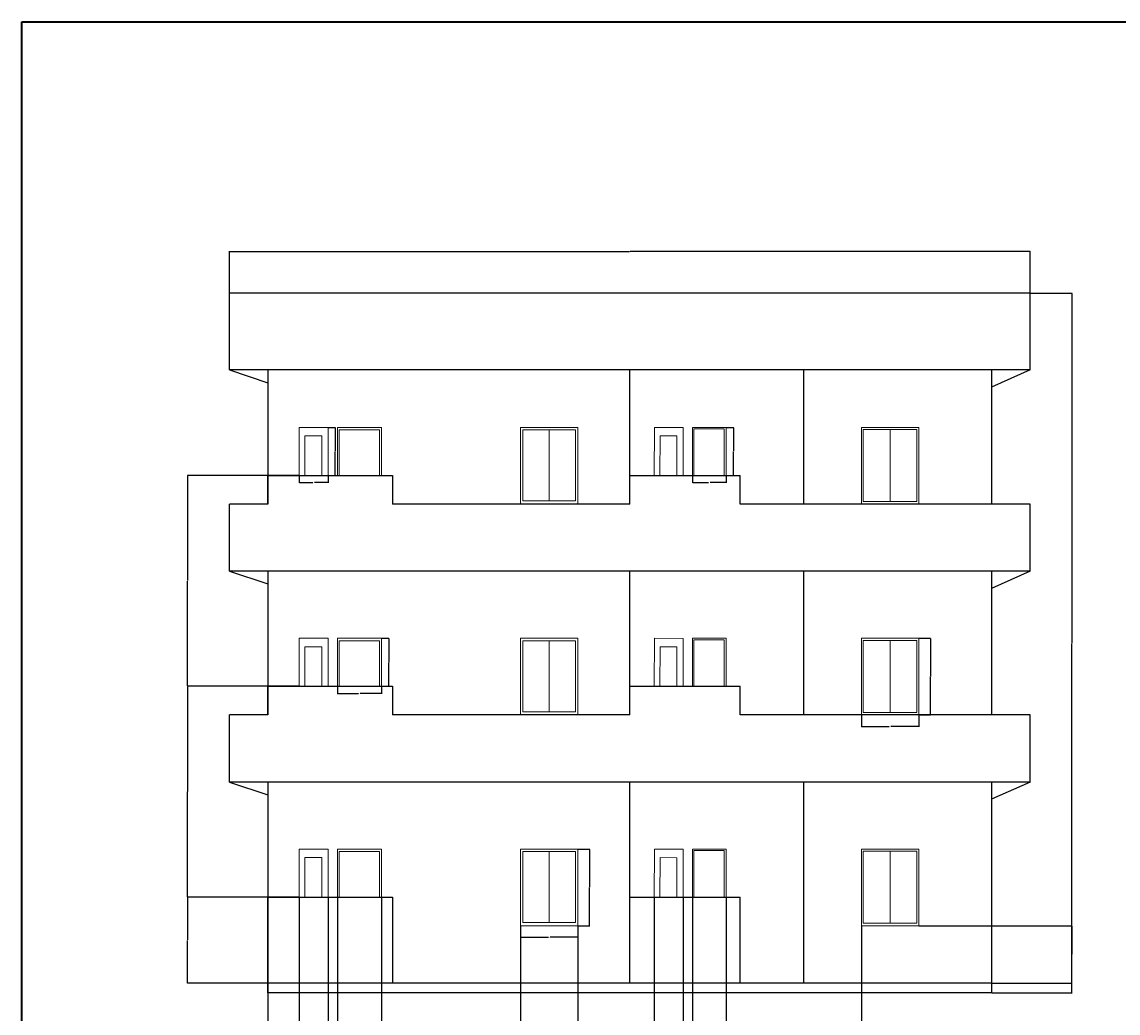
# Model space of a CAD drawing. Units: inches. Extents: x 2250 to 3629, y 982 to 2740.
# Tile 11 of 12: x 2250 to 2936, y 2119 to 2740. Entities that reach past the tile are written whole.
import ezdxf

# ---------------------------------------------------------------- set-up
doc = ezdxf.new("R2010")
doc.units = ezdxf.units.IN
for name, color, linetype, lineweight in [('A-ANNO-DIMS', 2, 'Continuous', 18), ('A-ANNO-TTLB', 7, 'Continuous', 35), ('A-ELEV', 7, 'Continuous', 25), ('A-ELEV-DOOR', 3, 'Continuous', 18), ('A-ELEV-GLAZ', 4, 'Continuous', 18)]:
    doc.layers.add(name, color=color, linetype=linetype, lineweight=lineweight)
doc.styles.get("Standard").update_dxf_attribs({"font": 'arial.ttf'})
doc.dimstyles.get("Standard").update_dxf_attribs({"dimtxt": 0.18, "dimasz": 0.18, "dimexe": 0.18, "dimexo": 0.0625, "dimgap": 0.09, "dimtad": 0, "dimtih": 1, "dimtoh": 1, "dimdec": 4, "dimzin": 0, "dimdsep": 46, "dimtxsty": 'Standard', "dimcen": 0.09, "dimadec": 0, "dimazin": 0, "dimtfac": 1, "dimtdec": 4, "dimtofl": 0, "dimtmove": 0, "dimatfit": 3, "dimfxl": 1, "dimtolj": 1, "dimtzin": 0, "dimarcsym": 0})

# ---------------------------------------------------------------- blocks, each defined once
blk = doc.blocks.new('EL-DOOR-18p04x30')
for p, q in [((0, 30), (0, 0)), ((18.04, 30), (0, 30)), ((18.04, 30), (18.04, 0))]:
    blk.add_line(p, q)
blk.add_lwpolyline([(3.53, 0), (3.53, 24.67), (14.13, 24.67), (14.13, 0)])
blk = doc.blocks.new('EL-WIN-27p64x30')
for p, q in [((0, 30), (0, 0)), ((27.64, 30), (0, 30)), ((27.64, 30), (27.64, 0))]:
    blk.add_line(p, q)
blk.add_lwpolyline([(1.16, 0), (1.16, 28.46), (26.36, 28.46), (26.36, 0)])
blk = doc.blocks.new('EL-WIN-36x48-A')
for p, q in [((0, 48), (0, 0)), ((36, 48), (0, 48)), ((17.95, 2), (17.95, 46.41)), ((36, 48), (36, 0)), ((36, 0), (0, 0))]:
    blk.add_line(p, q)
blk.add_lwpolyline([(1.44, 46.41), (34.46, 46.41), (34.46, 2), (1.44, 2)], close=True)
blk = doc.blocks.new('EL-WIN-21p24x30')
for p, q in [((0, 30), (0, 0)), ((21.23, 30), (0, 30)), ((0, 0), (0, 30)), ((21.23, 30), (21.23, 0)), ((21.23, 0), (21.23, 30))]:
    blk.add_line(p, q)
blk.add_lwpolyline([(0.82, 0), (0.82, 29.09), (19.98, 29.09), (19.98, 0)])
blk = doc.blocks.new('EL-WIN-36x48-B')
for p, q in [((0, 48), (0, 0)), ((36, 48), (0, 48)), ((17.97, 1.54), (17.97, 46.64)), ((36, 48), (36, 0)), ((36, 0), (0, 0))]:
    blk.add_line(p, q)
blk.add_lwpolyline([(1.24, 46.64), (34.71, 46.64), (34.71, 1.54), (1.24, 1.54)], close=True)
blk = doc.blocks.new('*D147')
at = {"layer": 'A-ANNO-DIMS', "color": 0, "lineweight": -2, "transparency": 16777216}
for p, q in [((2441.39, 2485.7), (2446.01, 2485.7)), ((2445.83, 2485.52), (2445.83, 2470.88)), ((2445.83, 2455.88), (2445.83, 2470.52)), ((2441.39, 2455.7), (2446.01, 2455.7))]:
    blk.add_line(p, q, dxfattribs=at)
at = {"layer": 'A-ANNO-DIMS', "color": 0, "transparency": 16777216}
for points in [[(2445.8, 2485.52), (2445.86, 2485.52), (2445.83, 2485.7)], [(2445.8, 2455.88), (2445.86, 2455.88), (2445.83, 2455.7)]]:
    blk.add_solid(points, dxfattribs=at)
at = {"layer": 'Defpoints', "color": 0, "transparency": 16777216}
for p in [(2441.33, 2485.7), (2445.83, 2485.7), (2441.33, 2455.7)]:
    blk.add_point(p, dxfattribs=at)
at = {"layer": 'A-ANNO-DIMS', "color": 0, "transparency": 16777216, "insert": (2445.83, 2470.7), "char_height": 0.18, "attachment_point": 5}
blk.add_mtext('\\A1;DOOR 30 TYP.', dxfattribs=at)
blk = doc.blocks.new('*D148')
at = {"layer": 'A-ANNO-DIMS', "color": 0, "lineweight": -2, "transparency": 16777216}
for p, q in [((2423.28, 2455.64), (2423.28, 2451.02)), ((2423.46, 2451.2), (2431.78, 2451.2)), ((2441.15, 2451.2), (2432.82, 2451.2)), ((2441.33, 2455.64), (2441.33, 2451.02))]:
    blk.add_line(p, q, dxfattribs=at)
at = {"layer": 'A-ANNO-DIMS', "color": 0, "transparency": 16777216}
for points in [[(2423.46, 2451.23), (2423.46, 2451.17), (2423.28, 2451.2)], [(2441.15, 2451.23), (2441.15, 2451.17), (2441.33, 2451.2)]]:
    blk.add_solid(points, dxfattribs=at)
at = {"layer": 'Defpoints', "color": 0, "transparency": 16777216}
for p in [(2423.28, 2455.7), (2441.33, 2455.7), (2441.33, 2451.2)]:
    blk.add_point(p, dxfattribs=at)
at = {"layer": 'A-ANNO-DIMS', "color": 0, "transparency": 16777216, "insert": (2432.3, 2451.2), "char_height": 0.18, "attachment_point": 5}
blk.add_mtext('\\A1;18 TYP.', dxfattribs=at)
blk = doc.blocks.new('*D149')
at = {"layer": 'A-ANNO-DIMS', "color": 0, "lineweight": -2, "transparency": 16777216}
for p, q in [((2474.81, 2353.7), (2479.42, 2353.7)), ((2479.24, 2353.52), (2479.24, 2338.88)), ((2479.24, 2323.88), (2479.24, 2338.52)), ((2474.81, 2323.7), (2479.42, 2323.7))]:
    blk.add_line(p, q, dxfattribs=at)
at = {"layer": 'A-ANNO-DIMS', "color": 0, "transparency": 16777216}
for points in [[(2479.21, 2353.52), (2479.27, 2353.52), (2479.24, 2353.7)], [(2479.21, 2323.88), (2479.27, 2323.88), (2479.24, 2323.7)]]:
    blk.add_solid(points, dxfattribs=at)
at = {"layer": 'Defpoints', "color": 0, "transparency": 16777216}
for p in [(2474.74, 2353.7), (2479.24, 2353.7), (2474.74, 2323.7)]:
    blk.add_point(p, dxfattribs=at)
at = {"layer": 'A-ANNO-DIMS', "color": 0, "transparency": 16777216, "insert": (2479.24, 2338.7), "char_height": 0.18, "attachment_point": 5}
blk.add_mtext('\\A1;WINDOW 30 TYP.', dxfattribs=at)
blk = doc.blocks.new('*D150')
at = {"layer": 'A-ANNO-DIMS', "color": 0, "lineweight": -2, "transparency": 16777216}
for p, q in [((2447.11, 2323.64), (2447.11, 2319.02)), ((2447.29, 2319.2), (2460.4, 2319.2)), ((2474.56, 2319.2), (2461.46, 2319.2)), ((2474.74, 2323.64), (2474.74, 2319.02))]:
    blk.add_line(p, q, dxfattribs=at)
at = {"layer": 'A-ANNO-DIMS', "color": 0, "transparency": 16777216}
for points in [[(2447.29, 2319.23), (2447.29, 2319.17), (2447.11, 2319.2)], [(2474.56, 2319.23), (2474.56, 2319.17), (2474.74, 2319.2)]]:
    blk.add_solid(points, dxfattribs=at)
at = {"layer": 'Defpoints', "color": 0, "transparency": 16777216}
for p in [(2447.11, 2323.7), (2474.74, 2323.7), (2474.74, 2319.2)]:
    blk.add_point(p, dxfattribs=at)
at = {"layer": 'A-ANNO-DIMS', "color": 0, "transparency": 16777216, "insert": (2460.93, 2319.2), "char_height": 0.18, "attachment_point": 5}
blk.add_mtext('\\A1;28 TYP.', dxfattribs=at)
blk = doc.blocks.new('*D151')
at = {"layer": 'A-ANNO-DIMS', "color": 0, "lineweight": -2, "transparency": 16777216}
for p, q in [((2597.75, 2221.7), (2605.07, 2221.7)), ((2604.89, 2221.52), (2604.89, 2197.88)), ((2604.89, 2173.88), (2604.89, 2197.52)), ((2597.75, 2173.7), (2605.07, 2173.7))]:
    blk.add_line(p, q, dxfattribs=at)
at = {"layer": 'A-ANNO-DIMS', "color": 0, "transparency": 16777216}
for points in [[(2604.86, 2221.52), (2604.92, 2221.52), (2604.89, 2221.7)], [(2604.86, 2173.88), (2604.92, 2173.88), (2604.89, 2173.7)]]:
    blk.add_solid(points, dxfattribs=at)
at = {"layer": 'Defpoints', "color": 0, "transparency": 16777216}
for p in [(2597.69, 2221.7), (2604.89, 2221.7), (2597.69, 2173.7)]:
    blk.add_point(p, dxfattribs=at)
at = {"layer": 'A-ANNO-DIMS', "color": 0, "transparency": 16777216, "insert": (2604.89, 2197.7), "char_height": 0.18, "attachment_point": 5}
blk.add_mtext('\\A1;WINDOW 48 TYP.', dxfattribs=at)
blk = doc.blocks.new('*D152')
at = {"layer": 'A-ANNO-DIMS', "color": 0, "lineweight": -2, "transparency": 16777216}
for p, q in [((2561.69, 2173.64), (2561.69, 2166.32)), ((2597.69, 2173.64), (2597.69, 2166.32)), ((2561.87, 2166.5), (2579.16, 2166.5)), ((2597.51, 2166.5), (2580.22, 2166.5))]:
    blk.add_line(p, q, dxfattribs=at)
at = {"layer": 'A-ANNO-DIMS', "color": 0, "transparency": 16777216}
for points in [[(2561.87, 2166.53), (2561.87, 2166.47), (2561.69, 2166.5)], [(2597.51, 2166.53), (2597.51, 2166.47), (2597.69, 2166.5)]]:
    blk.add_solid(points, dxfattribs=at)
at = {"layer": 'Defpoints', "color": 0, "transparency": 16777216}
for p in [(2561.69, 2173.7), (2597.69, 2173.7), (2597.69, 2166.5)]:
    blk.add_point(p, dxfattribs=at)
at = {"layer": 'A-ANNO-DIMS', "color": 0, "transparency": 16777216, "insert": (2579.69, 2166.5), "char_height": 0.18, "attachment_point": 5}
blk.add_mtext('\\A1;36 TYP.', dxfattribs=at)
blk = doc.blocks.new('*D153')
at = {"layer": 'A-ANNO-DIMS', "color": 0, "lineweight": -2, "transparency": 16777216}
for p, q in [((2690.61, 2485.7), (2695.22, 2485.7)), ((2695.04, 2485.52), (2695.04, 2470.88)), ((2695.04, 2455.88), (2695.04, 2470.52)), ((2690.61, 2455.7), (2695.22, 2455.7))]:
    blk.add_line(p, q, dxfattribs=at)
at = {"layer": 'A-ANNO-DIMS', "color": 0, "transparency": 16777216}
for points in [[(2695.01, 2485.52), (2695.07, 2485.52), (2695.04, 2485.7)], [(2695.01, 2455.88), (2695.07, 2455.88), (2695.04, 2455.7)]]:
    blk.add_solid(points, dxfattribs=at)
at = {"layer": 'Defpoints', "color": 0, "transparency": 16777216}
for p in [(2690.54, 2485.7), (2695.04, 2485.7), (2690.54, 2455.7)]:
    blk.add_point(p, dxfattribs=at)
at = {"layer": 'A-ANNO-DIMS', "color": 0, "transparency": 16777216, "insert": (2695.04, 2470.7), "char_height": 0.18, "attachment_point": 5}
blk.add_mtext('\\A1;WINDOW 30 TYP.', dxfattribs=at)
blk = doc.blocks.new('*D154')
at = {"layer": 'A-ANNO-DIMS', "color": 0, "lineweight": -2, "transparency": 16777216}
for p, q in [((2669.31, 2455.64), (2669.31, 2451.02)), ((2669.49, 2451.2), (2679.4, 2451.2)), ((2690.36, 2451.2), (2680.46, 2451.2)), ((2690.54, 2455.64), (2690.54, 2451.02))]:
    blk.add_line(p, q, dxfattribs=at)
at = {"layer": 'A-ANNO-DIMS', "color": 0, "transparency": 16777216}
for points in [[(2669.49, 2451.23), (2669.49, 2451.17), (2669.31, 2451.2)], [(2690.36, 2451.23), (2690.36, 2451.17), (2690.54, 2451.2)]]:
    blk.add_solid(points, dxfattribs=at)
at = {"layer": 'Defpoints', "color": 0, "transparency": 16777216}
for p in [(2669.31, 2455.7), (2690.54, 2455.7), (2690.54, 2451.2)]:
    blk.add_point(p, dxfattribs=at)
at = {"layer": 'A-ANNO-DIMS', "color": 0, "transparency": 16777216, "insert": (2679.93, 2451.2), "char_height": 0.18, "attachment_point": 5}
blk.add_mtext('\\A1;21 TYP.', dxfattribs=at)
blk = doc.blocks.new('*D155')
at = {"layer": 'A-ANNO-DIMS', "color": 0, "lineweight": -2, "transparency": 16777216}
for p, q in [((2811.11, 2353.7), (2818.43, 2353.7)), ((2818.25, 2353.52), (2818.25, 2329.88)), ((2818.25, 2305.88), (2818.25, 2329.52)), ((2811.11, 2305.7), (2818.43, 2305.7))]:
    blk.add_line(p, q, dxfattribs=at)
at = {"layer": 'A-ANNO-DIMS', "color": 0, "transparency": 16777216}
for points in [[(2818.22, 2353.52), (2818.28, 2353.52), (2818.25, 2353.7)], [(2818.22, 2305.88), (2818.28, 2305.88), (2818.25, 2305.7)]]:
    blk.add_solid(points, dxfattribs=at)
at = {"layer": 'Defpoints', "color": 0, "transparency": 16777216}
for p in [(2811.05, 2353.7), (2818.25, 2353.7), (2811.05, 2305.7)]:
    blk.add_point(p, dxfattribs=at)
at = {"layer": 'A-ANNO-DIMS', "color": 0, "transparency": 16777216, "insert": (2818.25, 2329.7), "char_height": 0.18, "attachment_point": 5}
blk.add_mtext('\\A1;WINDOW 48 TYP.', dxfattribs=at)
blk = doc.blocks.new('*D156')
at = {"layer": 'A-ANNO-DIMS', "color": 0, "lineweight": -2, "transparency": 16777216}
for p, q in [((2775.05, 2305.64), (2775.05, 2298.32)), ((2811.05, 2305.64), (2811.05, 2298.32)), ((2775.23, 2298.5), (2792.52, 2298.5)), ((2810.87, 2298.5), (2793.58, 2298.5))]:
    blk.add_line(p, q, dxfattribs=at)
at = {"layer": 'A-ANNO-DIMS', "color": 0, "transparency": 16777216}
for points in [[(2775.23, 2298.53), (2775.23, 2298.47), (2775.05, 2298.5)], [(2810.87, 2298.53), (2810.87, 2298.47), (2811.05, 2298.5)]]:
    blk.add_solid(points, dxfattribs=at)
at = {"layer": 'Defpoints', "color": 0, "transparency": 16777216}
for p in [(2775.05, 2305.7), (2811.05, 2305.7), (2811.05, 2298.5)]:
    blk.add_point(p, dxfattribs=at)
at = {"layer": 'A-ANNO-DIMS', "color": 0, "transparency": 16777216, "insert": (2793.05, 2298.5), "char_height": 0.18, "attachment_point": 5}
blk.add_mtext('\\A1;36 TYP.', dxfattribs=at)
blk = doc.blocks.new('*D176')
at = {"layer": 'A-ANNO-DIMS', "color": 0, "lineweight": -2, "transparency": 16777216}
for p, q in [((2379.61, 2569.76), (2379.61, 2596.08)), ((2379.79, 2595.9), (2629.84, 2595.9)), ((2880.43, 2595.9), (2630.38, 2595.9)), ((2880.61, 2569.76), (2880.61, 2596.08))]:
    blk.add_line(p, q, dxfattribs=at)
at = {"layer": 'A-ANNO-DIMS', "color": 0, "transparency": 16777216}
for points in [[(2379.79, 2595.93), (2379.79, 2595.87), (2379.61, 2595.9)], [(2880.43, 2595.93), (2880.43, 2595.87), (2880.61, 2595.9)]]:
    blk.add_solid(points, dxfattribs=at)
at = {"layer": 'Defpoints', "color": 0, "transparency": 16777216}
for p in [(2880.61, 2595.9), (2379.61, 2569.7), (2880.61, 2569.7)]:
    blk.add_point(p, dxfattribs=at)
at = {"layer": 'A-ANNO-DIMS', "color": 0, "transparency": 16777216, "insert": (2630.11, 2595.9), "char_height": 0.18, "attachment_point": 5}
blk.add_mtext('\\A1;501', dxfattribs=at)
blk = doc.blocks.new('*D177')
at = {"layer": 'A-ANNO-DIMS', "color": 0, "lineweight": -2, "transparency": 16777216}
for p, q in [((2880.67, 2569.7), (2906.99, 2569.7)), ((2906.81, 2569.52), (2906.81, 2350.88)), ((2906.81, 2131.88), (2906.81, 2350.52)), ((2856.67, 2131.7), (2906.99, 2131.7))]:
    blk.add_line(p, q, dxfattribs=at)
at = {"layer": 'A-ANNO-DIMS', "color": 0, "transparency": 16777216}
for points in [[(2906.78, 2569.52), (2906.84, 2569.52), (2906.81, 2569.7)], [(2906.78, 2131.88), (2906.84, 2131.88), (2906.81, 2131.7)]]:
    blk.add_solid(points, dxfattribs=at)
at = {"layer": 'Defpoints', "color": 0, "transparency": 16777216}
for p in [(2880.61, 2569.7), (2906.81, 2569.7), (2856.61, 2131.7)]:
    blk.add_point(p, dxfattribs=at)
at = {"layer": 'A-ANNO-DIMS', "color": 0, "transparency": 16777216, "insert": (2906.81, 2350.7), "char_height": 0.18, "attachment_point": 5}
blk.add_mtext('\\A1;438', dxfattribs=at)
blk = doc.blocks.new('*D178')
at = {"layer": 'A-ANNO-DIMS', "color": 0, "lineweight": -2, "transparency": 16777216}
for p, q in [((2423.22, 2191.7), (2353.23, 2191.7)), ((2353.41, 2191.52), (2353.41, 2164.88)), ((2353.41, 2137.88), (2353.41, 2164.52)), ((2403.54, 2137.7), (2353.23, 2137.7))]:
    blk.add_line(p, q, dxfattribs=at)
at = {"layer": 'A-ANNO-DIMS', "color": 0, "transparency": 16777216}
for points in [[(2353.38, 2191.52), (2353.44, 2191.52), (2353.41, 2191.7)], [(2353.38, 2137.88), (2353.44, 2137.88), (2353.41, 2137.7)]]:
    blk.add_solid(points, dxfattribs=at)
at = {"layer": 'Defpoints', "color": 0, "transparency": 16777216}
for p in [(2353.41, 2191.7), (2423.28, 2191.7), (2403.61, 2137.7)]:
    blk.add_point(p, dxfattribs=at)
at = {"layer": 'A-ANNO-DIMS', "color": 0, "transparency": 16777216, "insert": (2353.41, 2164.7), "char_height": 0.18, "attachment_point": 5}
blk.add_mtext('\\A1;54', dxfattribs=at)
blk = doc.blocks.new('*D179')
at = {"layer": 'A-ANNO-DIMS', "color": 0, "lineweight": -2, "transparency": 16777216}
for p, q in [((2423.22, 2323.7), (2353.23, 2323.7)), ((2353.41, 2323.52), (2353.41, 2257.88)), ((2353.41, 2191.88), (2353.41, 2257.52)), ((2423.22, 2191.7), (2353.23, 2191.7))]:
    blk.add_line(p, q, dxfattribs=at)
at = {"layer": 'A-ANNO-DIMS', "color": 0, "transparency": 16777216}
for points in [[(2353.38, 2323.52), (2353.44, 2323.52), (2353.41, 2323.7)], [(2353.38, 2191.88), (2353.44, 2191.88), (2353.41, 2191.7)]]:
    blk.add_solid(points, dxfattribs=at)
at = {"layer": 'Defpoints', "color": 0, "transparency": 16777216}
for p in [(2353.41, 2323.7), (2423.28, 2323.7), (2423.28, 2191.7)]:
    blk.add_point(p, dxfattribs=at)
at = {"layer": 'A-ANNO-DIMS', "color": 0, "transparency": 16777216, "insert": (2353.41, 2257.7), "char_height": 0.18, "attachment_point": 5}
blk.add_mtext('\\A1;132', dxfattribs=at)
blk = doc.blocks.new('*D180')
at = {"layer": 'A-ANNO-DIMS', "color": 0, "lineweight": -2, "transparency": 16777216}
for p, q in [((2423.22, 2455.7), (2353.23, 2455.7)), ((2353.41, 2455.52), (2353.41, 2389.88)), ((2353.41, 2323.88), (2353.41, 2389.52)), ((2423.22, 2323.7), (2353.23, 2323.7))]:
    blk.add_line(p, q, dxfattribs=at)
at = {"layer": 'A-ANNO-DIMS', "color": 0, "transparency": 16777216}
for points in [[(2353.38, 2455.52), (2353.44, 2455.52), (2353.41, 2455.7)], [(2353.38, 2323.88), (2353.44, 2323.88), (2353.41, 2323.7)]]:
    blk.add_solid(points, dxfattribs=at)
at = {"layer": 'Defpoints', "color": 0, "transparency": 16777216}
for p in [(2353.41, 2455.7), (2423.28, 2455.7), (2423.28, 2323.7)]:
    blk.add_point(p, dxfattribs=at)
at = {"layer": 'A-ANNO-DIMS', "color": 0, "transparency": 16777216, "insert": (2353.41, 2389.7), "char_height": 0.18, "attachment_point": 5}
blk.add_mtext('\\A1;132', dxfattribs=at)
blk = doc.blocks.new('*D181')
at = {"layer": 'A-ANNO-DIMS', "color": 0, "lineweight": -2, "transparency": 16777216}
for p, q in [((2423.28, 2191.64), (2423.28, 2061.34)), ((2403.61, 2131.64), (2403.61, 2061.34)), ((2403.79, 2061.52), (2412.99, 2061.52)), ((2423.1, 2061.52), (2413.9, 2061.52))]:
    blk.add_line(p, q, dxfattribs=at)
at = {"layer": 'A-ANNO-DIMS', "color": 0, "transparency": 16777216}
for points in [[(2403.79, 2061.55), (2403.79, 2061.49), (2403.61, 2061.52)], [(2423.1, 2061.55), (2423.1, 2061.49), (2423.28, 2061.52)]]:
    blk.add_solid(points, dxfattribs=at)
at = {"layer": 'Defpoints', "color": 0, "transparency": 16777216}
for p in [(2423.28, 2191.7), (2403.61, 2131.7), (2423.28, 2061.52)]:
    blk.add_point(p, dxfattribs=at)
at = {"layer": 'A-ANNO-DIMS', "color": 0, "transparency": 16777216, "insert": (2413.44, 2061.52), "char_height": 0.18, "attachment_point": 5}
blk.add_mtext('\\A1;19.674', dxfattribs=at)
blk = doc.blocks.new('*D182')
at = {"layer": 'A-ANNO-DIMS', "color": 0, "lineweight": -2, "transparency": 16777216}
for p, q in [((2441.33, 2191.64), (2441.33, 2061.34)), ((2447.11, 2191.64), (2447.11, 2061.34)), ((2441.51, 2061.52), (2443.84, 2061.52)), ((2446.93, 2061.52), (2444.59, 2061.52))]:
    blk.add_line(p, q, dxfattribs=at)
at = {"layer": 'A-ANNO-DIMS', "color": 0, "transparency": 16777216}
for points in [[(2441.51, 2061.55), (2441.51, 2061.49), (2441.33, 2061.52)], [(2446.93, 2061.55), (2446.93, 2061.49), (2447.11, 2061.52)]]:
    blk.add_solid(points, dxfattribs=at)
at = {"layer": 'Defpoints', "color": 0, "transparency": 16777216}
for p in [(2441.33, 2191.7), (2447.11, 2191.7), (2447.11, 2061.52)]:
    blk.add_point(p, dxfattribs=at)
at = {"layer": 'A-ANNO-DIMS', "color": 0, "transparency": 16777216, "insert": (2444.22, 2061.52), "char_height": 0.18, "attachment_point": 5}
blk.add_mtext('\\A1;5.781', dxfattribs=at)
blk = doc.blocks.new('*D183')
at = {"layer": 'A-ANNO-DIMS', "color": 0, "lineweight": -2, "transparency": 16777216}
for p, q in [((2474.74, 2191.64), (2474.74, 2061.34)), ((2561.69, 2173.64), (2561.69, 2061.34)), ((2474.92, 2061.52), (2517.82, 2061.52)), ((2561.51, 2061.52), (2518.61, 2061.52))]:
    blk.add_line(p, q, dxfattribs=at)
at = {"layer": 'A-ANNO-DIMS', "color": 0, "transparency": 16777216}
for points in [[(2474.92, 2061.55), (2474.92, 2061.49), (2474.74, 2061.52)], [(2561.51, 2061.55), (2561.51, 2061.49), (2561.69, 2061.52)]]:
    blk.add_solid(points, dxfattribs=at)
at = {"layer": 'Defpoints', "color": 0, "transparency": 16777216}
for p in [(2474.74, 2191.7), (2561.69, 2173.7), (2561.69, 2061.52)]:
    blk.add_point(p, dxfattribs=at)
at = {"layer": 'A-ANNO-DIMS', "color": 0, "transparency": 16777216, "insert": (2518.22, 2061.52), "char_height": 0.18, "attachment_point": 5}
blk.add_mtext('\\A1;86.94', dxfattribs=at)
blk = doc.blocks.new('*D184')
at = {"layer": 'A-ANNO-DIMS', "color": 0, "lineweight": -2, "transparency": 16777216}
for p, q in [((2645.41, 2191.68), (2645.41, 2061.34)), ((2597.69, 2173.64), (2597.69, 2061.34)), ((2597.87, 2061.52), (2621.08, 2061.52)), ((2645.23, 2061.52), (2622.02, 2061.52))]:
    blk.add_line(p, q, dxfattribs=at)
at = {"layer": 'A-ANNO-DIMS', "color": 0, "transparency": 16777216}
for points in [[(2597.87, 2061.55), (2597.87, 2061.49), (2597.69, 2061.52)], [(2645.23, 2061.55), (2645.23, 2061.49), (2645.41, 2061.52)]]:
    blk.add_solid(points, dxfattribs=at)
at = {"layer": 'Defpoints', "color": 0, "transparency": 16777216}
for p in [(2645.41, 2191.74), (2597.69, 2173.7), (2645.41, 2061.52)]:
    blk.add_point(p, dxfattribs=at)
at = {"layer": 'A-ANNO-DIMS', "color": 0, "transparency": 16777216, "insert": (2621.55, 2061.52), "char_height": 0.18, "attachment_point": 5}
blk.add_mtext('\\A1;47.725', dxfattribs=at)
blk = doc.blocks.new('*D185')
at = {"layer": 'A-ANNO-DIMS', "color": 0, "lineweight": -2, "transparency": 16777216}
for p, q in [((2663.46, 2191.6), (2663.46, 2061.34)), ((2669.31, 2191.64), (2669.31, 2061.34)), ((2663.64, 2061.52), (2666.06, 2061.52)), ((2669.13, 2061.52), (2666.71, 2061.52))]:
    blk.add_line(p, q, dxfattribs=at)
at = {"layer": 'A-ANNO-DIMS', "color": 0, "transparency": 16777216}
for points in [[(2663.64, 2061.55), (2663.64, 2061.49), (2663.46, 2061.52)], [(2669.13, 2061.55), (2669.13, 2061.49), (2669.31, 2061.52)]]:
    blk.add_solid(points, dxfattribs=at)
at = {"layer": 'Defpoints', "color": 0, "transparency": 16777216}
for p in [(2663.46, 2191.66), (2669.31, 2191.7), (2669.31, 2061.52)]:
    blk.add_point(p, dxfattribs=at)
at = {"layer": 'A-ANNO-DIMS', "color": 0, "transparency": 16777216, "insert": (2666.38, 2061.52), "char_height": 0.18, "attachment_point": 5}
blk.add_mtext('\\A1;5.85', dxfattribs=at)
blk = doc.blocks.new('*D186')
at = {"layer": 'A-ANNO-DIMS', "color": 0, "lineweight": -2, "transparency": 16777216}
for p, q in [((2690.54, 2191.64), (2690.54, 2061.34)), ((2775.05, 2173.64), (2775.05, 2061.34)), ((2690.72, 2061.52), (2732.47, 2061.52)), ((2774.87, 2061.52), (2733.12, 2061.52))]:
    blk.add_line(p, q, dxfattribs=at)
at = {"layer": 'A-ANNO-DIMS', "color": 0, "transparency": 16777216}
for points in [[(2690.72, 2061.55), (2690.72, 2061.49), (2690.54, 2061.52)], [(2774.87, 2061.55), (2774.87, 2061.49), (2775.05, 2061.52)]]:
    blk.add_solid(points, dxfattribs=at)
at = {"layer": 'Defpoints', "color": 0, "transparency": 16777216}
for p in [(2690.54, 2191.7), (2775.05, 2173.7), (2775.05, 2061.52)]:
    blk.add_point(p, dxfattribs=at)
at = {"layer": 'A-ANNO-DIMS', "color": 0, "transparency": 16777216, "insert": (2732.8, 2061.52), "char_height": 0.18, "attachment_point": 5}
blk.add_mtext('\\A1;84.5', dxfattribs=at)
blk = doc.blocks.new('*D187')
at = {"layer": 'A-ANNO-DIMS', "color": 0, "lineweight": -2, "transparency": 16777216}
for p, q in [((2811.11, 2173.7), (2906.99, 2173.7)), ((2906.81, 2173.52), (2906.81, 2155.88)), ((2906.81, 2137.88), (2906.81, 2155.52)), ((2856.67, 2137.7), (2906.99, 2137.7))]:
    blk.add_line(p, q, dxfattribs=at)
at = {"layer": 'A-ANNO-DIMS', "color": 0, "transparency": 16777216}
for points in [[(2906.78, 2173.52), (2906.84, 2173.52), (2906.81, 2173.7)], [(2906.78, 2137.88), (2906.84, 2137.88), (2906.81, 2137.7)]]:
    blk.add_solid(points, dxfattribs=at)
at = {"layer": 'Defpoints', "color": 0, "transparency": 16777216}
for p in [(2811.05, 2173.7), (2906.81, 2173.7), (2856.61, 2137.7)]:
    blk.add_point(p, dxfattribs=at)
at = {"layer": 'A-ANNO-DIMS', "color": 0, "transparency": 16777216, "insert": (2906.81, 2155.7), "char_height": 0.18, "attachment_point": 5}
blk.add_mtext('\\A1;36', dxfattribs=at)

msp = doc.modelspace()

# ---------------------------------------------------------------- linework, layer by layer
at = {"layer": 'A-ANNO-TTLB'}
msp.add_lwpolyline([(2249.6849, 2739.593), (3629.4532, 2739.593), (3629.4532, 982.3108), (2249.6849, 982.3108)], close=True, dxfattribs=at)
at = {"layer": 'A-ELEV'}
for p, q in [((2880.6072, 2569.6999), (2379.6072, 2569.6999)), ((2379.6072, 2521.6999), (2379.6072, 2569.6999)), ((2880.6072, 2521.6999), (2880.6072, 2569.6999)), ((2880.6072, 2521.6999), (2379.6072, 2521.6999)), ((2379.6072, 2521.6999), (2403.6072, 2513.7231)), ((2403.6072, 2521.6999), (2403.6072, 2437.6999)), ((2630.1072, 2437.6999), (2630.1072, 2521.6999)), ((2739.0543, 2437.6999), (2739.0543, 2521.6999)), ((2856.6072, 2521.6999), (2856.6072, 2437.6999)), ((2880.6072, 2521.6999), (2856.6072, 2510.907)), ((2403.6072, 2437.6999), (2403.6072, 2455.6999)), ((2403.6072, 2455.6999), (2481.6072, 2455.6999)), ((2481.6072, 2455.6999), (2481.6072, 2437.6999)), ((2630.1072, 2455.6999), (2690.5428, 2455.6999)), ((2690.5428, 2455.6999), (2699.1258, 2455.6999)), ((2699.1258, 2437.6999), (2699.1258, 2455.6999)), ((2403.6072, 2437.6999), (2379.6072, 2437.6999)), ((2379.6072, 2395.6999), (2379.6072, 2437.6999)), ((2630.1072, 2437.6999), (2481.6072, 2437.6999)), ((2880.6072, 2437.6999), (2699.1258, 2437.6999)), ((2880.6072, 2395.6999), (2880.6072, 2437.6999)), ((2880.6072, 2395.6999), (2379.6072, 2395.6999)), ((2379.6072, 2395.6999), (2403.6072, 2387.7231)), ((2403.6072, 2395.6999), (2403.6072, 2305.6999)), ((2630.1072, 2305.6999), (2630.1072, 2395.6999)), ((2739.0543, 2305.6999), (2739.0543, 2395.6999)), ((2856.6072, 2395.6999), (2856.6072, 2305.6999)), ((2880.6072, 2395.6999), (2856.6072, 2384.907)), ((2403.6072, 2305.6999), (2403.6072, 2323.6999)), ((2403.6072, 2323.6999), (2481.6072, 2323.6999)), ((2481.6072, 2323.6999), (2481.6072, 2305.6999)), ((2630.1072, 2323.6999), (2690.5428, 2323.6999)), ((2690.5428, 2323.6999), (2699.1258, 2323.6999)), ((2699.1258, 2305.6999), (2699.1258, 2323.6999)), ((2379.6072, 2263.6999), (2379.6072, 2305.6999)), ((2403.6072, 2305.6999), (2379.6072, 2305.6999)), ((2630.1072, 2305.6999), (2481.6072, 2305.6999)), ((2880.6072, 2305.6999), (2699.1258, 2305.6999)), ((2880.6072, 2263.6999), (2880.6072, 2305.6999)), ((2880.6072, 2263.6999), (2379.6072, 2263.6999)), ((2379.6072, 2263.6999), (2403.6072, 2255.7231)), ((2403.6072, 2263.6999), (2403.6072, 2131.6999)), ((2630.1072, 2137.6999), (2630.1072, 2263.6999)), ((2739.0543, 2137.6999), (2739.0543, 2263.6999)), ((2856.6072, 2263.6999), (2856.6072, 2131.6999)), ((2880.6072, 2263.6999), (2856.6072, 2252.907)), ((2403.6072, 2131.6999), (2403.6072, 2191.6999)), ((2403.6072, 2191.6999), (2481.6072, 2191.6999)), ((2481.6072, 2191.6999), (2481.6072, 2137.6999)), ((2630.1072, 2191.6999), (2690.5428, 2191.6999)), ((2690.5428, 2191.6999), (2699.1258, 2191.6999)), ((2699.1258, 2137.6999), (2699.1258, 2191.6999)), ((2856.6072, 2137.6999), (2403.6072, 2137.6999)), ((2856.6072, 2131.6999), (2403.6072, 2131.6999))]:
    msp.add_line(p, q, dxfattribs=at)

# ---------------------------------------------------------------- block references
at = {"layer": 'A-ELEV-DOOR'}
for p in [(2423.282, 2455.7), (2423.282, 2323.7), (2423.282, 2191.7)]:
    msp.add_blockref('EL-DOOR-18p04x30', p, dxfattribs=at)
for p, rotation in [((2645.4146, 2455.7388), 359.7526193396808), ((2645.4146, 2323.7388), 359.7526193396808), ((2645.4146, 2191.7388), 359.7526193396837)]:
    msp.add_blockref('EL-DOOR-18p04x30', p, dxfattribs=dict(at, rotation=rotation))
at = {"layer": 'A-ELEV-GLAZ'}
for name, p in [('EL-WIN-27p64x30', (2447.107, 2455.7)), ('EL-WIN-36x48-A', (2561.689, 2437.7)), ('EL-WIN-21p24x30', (2669.308, 2455.7)), ('EL-WIN-36x48-B', (2775.05, 2437.7)), ('EL-WIN-27p64x30', (2447.107, 2323.7)), ('EL-WIN-36x48-A', (2561.689, 2305.7)), ('EL-WIN-21p24x30', (2669.308, 2323.7)), ('EL-WIN-36x48-B', (2775.05, 2305.7)), ('EL-WIN-27p64x30', (2447.107, 2191.7)), ('EL-WIN-36x48-A', (2561.689, 2173.7)), ('EL-WIN-21p24x30', (2669.308, 2191.7)), ('EL-WIN-36x48-B', (2775.05, 2173.7))]:
    msp.add_blockref(name, p, dxfattribs=at)

# ---------------------------------------------------------------- dimensions: what is measured, and where the dimension line sits
at = {"layer": 'A-ANNO-DIMS'}
for base, p1, p2, override, picture, middle in [((2880.6072, 2595.8999), (2379.6072, 2569.6999), (2880.6072, 2569.6999), {"dimdec": 0, "dimlfac": 1, "dimrnd": 0, "dimzin": 0, "dimdsep": 46, "dimlunit": 2}, '*D176', (2630.1072, 2595.8999)), ((2423.2815, 2061.5229), (2403.6072, 2131.6999), (2423.2815, 2191.6999), {"dimdec": 3, "dimlfac": 1, "dimrnd": 0, "dimzin": 0, "dimdsep": 46, "dimlunit": 2}, '*D181', (2413.4444, 2061.5229)), ((2447.1072, 2061.5229), (2441.3258, 2191.6999), (2447.1072, 2191.6999), {"dimdec": 3, "dimlfac": 1, "dimrnd": 0, "dimzin": 0, "dimdsep": 46, "dimlunit": 2}, '*D182', (2444.2165, 2061.5229)), ((2561.6892, 2061.5229), (2474.7443, 2191.6999), (2561.6892, 2173.6999), {"dimdec": 2, "dimlfac": 1, "dimrnd": 0, "dimzin": 0, "dimdsep": 46, "dimlunit": 2}, '*D183', (2518.2168, 2061.5229)), ((2645.4141, 2061.5229), (2597.6892, 2173.6999), (2645.4141, 2191.7387), {"dimdec": 3, "dimlfac": 1, "dimrnd": 0, "dimzin": 0, "dimdsep": 46, "dimlunit": 2}, '*D184', (2621.5517, 2061.5229)), ((2669.3082, 2061.5229), (2663.4583, 2191.6608), (2669.3082, 2191.6999), {"dimdec": 2, "dimlfac": 1, "dimrnd": 0, "dimzin": 0, "dimdsep": 46, "dimlunit": 2}, '*D185', (2666.3832, 2061.5229)), ((2775.0497, 2061.5229), (2690.5428, 2191.6999), (2775.0497, 2173.6999), {"dimdec": 1, "dimlfac": 1, "dimrnd": 0, "dimzin": 0, "dimdsep": 46, "dimlunit": 2}, '*D186', (2732.7962, 2061.5229))]:
    dim = msp.add_linear_dim(base=base, p1=p1, p2=p2, dimstyle='Standard', override=override, dxfattribs=at)
    dim.commit()
    dim.dimension.update_dxf_attribs({"geometry": picture, "text_midpoint": middle})
for base, p1, p2, picture, middle in [((2906.8072, 2569.6999), (2856.6072, 2131.6999), (2880.6072, 2569.6999), '*D177', (2906.8072, 2350.6999)), ((2353.4072, 2455.6999), (2423.2815, 2323.6999), (2423.2815, 2455.6999), '*D180', (2353.4072, 2389.6999)), ((2353.4072, 2323.6999), (2423.2815, 2191.6999), (2423.2815, 2323.6999), '*D179', (2353.4072, 2257.6999)), ((2353.4072, 2191.6999), (2403.6072, 2137.6999), (2423.2815, 2191.6999), '*D178', (2353.4072, 2164.6999)), ((2906.8072, 2173.6999), (2856.6072, 2137.6999), (2811.0497, 2173.6999), '*D187', (2906.8072, 2155.6999))]:
    dim = msp.add_linear_dim(base=base, p1=p1, p2=p2, angle=90, dimstyle='Standard', override={"dimdec": 0, "dimlfac": 1, "dimrnd": 0, "dimzin": 0, "dimdsep": 46, "dimlunit": 2}, dxfattribs=at)
    dim.commit()
    dim.dimension.update_dxf_attribs({"geometry": picture, "text_midpoint": middle})
for base, p1, p2, text, picture, middle in [((2445.8258, 2485.6999), (2441.3258, 2455.6999), (2441.3258, 2485.6999), 'DOOR <> TYP.', '*D147', (2445.8258, 2470.6999)), ((2695.0428, 2485.6999), (2690.5428, 2455.6999), (2690.5428, 2485.6999), 'WINDOW <> TYP.', '*D153', (2695.0428, 2470.6999)), ((2479.2443, 2353.6999), (2474.7443, 2323.6999), (2474.7443, 2353.6999), 'WINDOW <> TYP.', '*D149', (2479.2443, 2338.6999)), ((2818.2497, 2353.6999), (2811.0497, 2305.6999), (2811.0497, 2353.6999), 'WINDOW <> TYP.', '*D155', (2818.2497, 2329.6999)), ((2604.8892, 2221.6999), (2597.6892, 2173.6999), (2597.6892, 2221.6999), 'WINDOW <> TYP.', '*D151', (2604.8892, 2197.6999))]:
    dim = msp.add_linear_dim(base=base, p1=p1, p2=p2, angle=90, text=text, dimstyle='Standard', override={"dimdec": 0, "dimlfac": 1, "dimrnd": 0, "dimzin": 0, "dimdsep": 46, "dimlunit": 2}, dxfattribs=at)
    dim.commit()
    dim.dimension.update_dxf_attribs({"geometry": picture, "text_midpoint": middle})
for base, p1, p2, picture, middle in [((2441.3258, 2451.1999), (2423.2815, 2455.6999), (2441.3258, 2455.6999), '*D148', (2432.3037, 2451.1999)), ((2690.5428, 2451.1999), (2669.3082, 2455.6999), (2690.5428, 2455.6999), '*D154', (2679.9255, 2451.1999)), ((2474.7443, 2319.1999), (2447.1072, 2323.6999), (2474.7443, 2323.6999), '*D150', (2460.9258, 2319.1999)), ((2811.0497, 2298.4999), (2775.0497, 2305.6999), (2811.0497, 2305.6999), '*D156', (2793.0497, 2298.4999)), ((2597.6892, 2166.4999), (2561.6892, 2173.6999), (2597.6892, 2173.6999), '*D152', (2579.6892, 2166.4999))]:
    dim = msp.add_linear_dim(base=base, p1=p1, p2=p2, text='<> TYP.', dimstyle='Standard', override={"dimdec": 0, "dimlfac": 1, "dimrnd": 0, "dimzin": 0, "dimdsep": 46, "dimlunit": 2}, dxfattribs=at)
    dim.commit()
    dim.dimension.update_dxf_attribs({"geometry": picture, "text_midpoint": middle})

doc.saveas('drawing.dxf')
